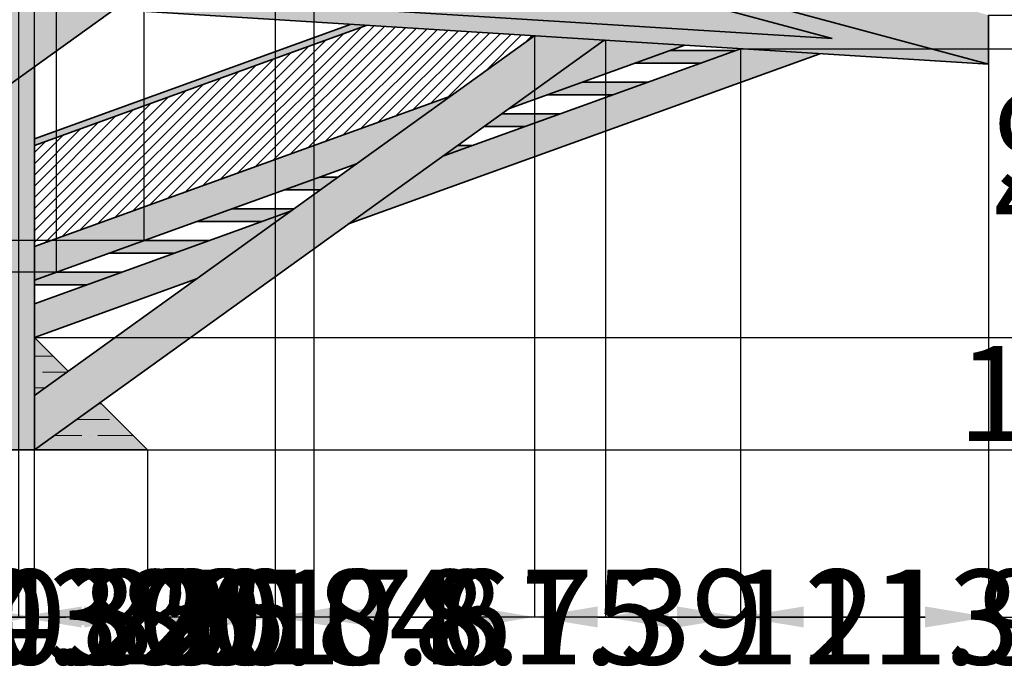
# Model space of a CAD drawing. Units: millimetres. Extents: x -504 to 6314, y 1290 to 4335.
# Tile 6 of 9: x 3796 to 5350, y 1290 to 2332. Entities that reach past the tile are written whole.
import ezdxf

# ---------------------------------------------------------------- set-up
doc = ezdxf.new("R2010")
doc.units = ezdxf.units.MM
doc.header["$MEASUREMENT"] = 0
for name, color, linetype, lineweight in [('A-ANNO-DIMS', 2, 'Continuous', 18), ('A-ELEV', 7, 'Continuous', 35), ('A-ELEV-PATT', 8, 'Continuous', 13)]:
    doc.layers.add(name, color=color, linetype=linetype, lineweight=lineweight)
doc.styles.get("Standard").update_dxf_attribs({"font": 'arial.ttf'})
doc.dimstyles.get("Standard").update_dxf_attribs({"dimtxt": 150, "dimasz": 100, "dimexe": 0.18, "dimexo": 0.0625, "dimgap": 0.09, "dimtad": 0, "dimtih": 1, "dimtoh": 1, "dimdec": 0, "dimzin": 0, "dimdsep": 46, "dimtxsty": 'Standard', "dimcen": 0.09, "dimadec": 0, "dimazin": 0, "dimtfac": 1, "dimtdec": 0, "dimtofl": 0, "dimtmove": 0, "dimatfit": 3, "dimfxl": 1, "dimtolj": 1, "dimtzin": 0, "dimarcsym": 0})
pattern_1 = [(50, (0, 0), (71.726, -6.2752), [7.5, -82.5]), (355, (0, 0), (-13.8751, 75.2192), [6, -66]), (100.4514, (5.98, -0.52), (57.8509, 68.944), [6.374, -70.1142]), (46.1842, (0, 20), (106.7241, -16.5519), [11.25, -123.75]), (96.6356, (8.89, 18.62), (93.4662, 97.4119), [9.561, -105.1714]), (351.1842, (0, 20), (93.4662, 97.4119), [9, -99]), (21, (10, 15), (59.6907, -40.2619), [7.5, -82.5]), (326, (10, 15), (24.3315, 72.515), [6, -66]), (71.4514, (14.974, 11.645), (84.0222, 32.2531), [6.374, -70.1142]), (37.5, (0, 0), (1.21599, 33.28939), [0, -65.2, 0, -67, 0, -66.25]), (7.5, (0, 0), (26.30695, 39.44117), [0, -38.2, 0, -63.7, 0, -25.25]), (327.5, (-22.3, 0), (53.38224, -2.25549), [0, -25, 0, -78, 0, -103.5]), (317.5, (-32.3, 0), (58.3186, 10.0105), [0, -32.5, 0, -51.8, 0, -73.5])]

# ---------------------------------------------------------------- blocks, each defined once
blk = doc.blocks.new('*D1')
at = {"layer": 'A-ANNO-DIMS', "color": 0, "lineweight": -2, "transparency": 16777216}
for p, q in [((5324.8, 2261.1), (5324.8, 1387.9)), ((72.8, 1652.1), (72.8, 1387.9)), ((172.8, 1388.1), (2475.5, 1388.1)), ((5224.8, 1388.1), (2922.1, 1388.1))]:
    blk.add_line(p, q, dxfattribs=at)
at = {"layer": 'A-ANNO-DIMS', "color": 0, "transparency": 16777216}
for points in [[(172.8, 1404.8), (172.8, 1371.5), (72.8, 1388.1)], [(5224.8, 1404.8), (5224.8, 1371.5), (5324.8, 1388.1)]]:
    blk.add_solid(points, dxfattribs=at)
at = {"layer": 'Defpoints', "color": 0, "transparency": 16777216}
for p in [(5324.8, 2261.2), (72.8, 1652.1), (5324.8, 1388.1)]:
    blk.add_point(p, dxfattribs=at)
at = {"layer": 'A-ANNO-DIMS', "color": 0, "transparency": 16777216, "insert": (2698.8, 1388.1), "char_height": 150, "attachment_point": 5}
blk.add_mtext('\\A1;5252', dxfattribs=at)
blk = doc.blocks.new('*D5')
at = {"layer": 'A-ANNO-DIMS', "color": 0, "lineweight": -2, "transparency": 16777216}
for p, q in [((4260.1, 2625.8), (5589, 2625.8)), ((5588.8, 2525.8), (5588.8, 2215.7)), ((5588.8, 1752.1), (5588.8, 2062.2)), ((72.9, 1652.1), (5589, 1652.1))]:
    blk.add_line(p, q, dxfattribs=at)
at = {"layer": 'A-ANNO-DIMS', "color": 0, "transparency": 16777216}
for points in [[(5572.1, 2525.8), (5605.5, 2525.8), (5588.8, 2625.8)], [(5572.1, 1752.1), (5605.5, 1752.1), (5588.8, 1652.1)]]:
    blk.add_solid(points, dxfattribs=at)
at = {"layer": 'Defpoints', "color": 0, "transparency": 16777216}
for p in [(4260, 2625.8), (5588.8, 2625.8), (72.8, 1652.1)]:
    blk.add_point(p, dxfattribs=at)
at = {"layer": 'A-ANNO-DIMS', "color": 0, "transparency": 16777216, "insert": (5588.8, 2138.9), "char_height": 150, "attachment_point": 5}
blk.add_mtext('\\A1;973.6', dxfattribs=at)
blk = doc.blocks.new('*D38')
at = {"layer": 'A-ANNO-DIMS', "color": 0, "lineweight": -2, "transparency": 16777216}
for p, q in [((2963.6, 2625.7), (2963.6, 1387.9)), ((3407.8, 2625.7), (3407.8, 1387.9)), ((3063.6, 1388.1), (3307.8, 1388.1)), ((3407.8, 1388.1), (3507.8, 1388.1))]:
    blk.add_line(p, q, dxfattribs=at)
at = {"layer": 'A-ANNO-DIMS', "color": 0, "transparency": 16777216}
for points in [[(3063.6, 1404.8), (3063.6, 1371.5), (2963.6, 1388.1)], [(3307.8, 1404.8), (3307.8, 1371.5), (3407.8, 1388.1)]]:
    blk.add_solid(points, dxfattribs=at)
at = {"layer": 'Defpoints', "color": 0, "transparency": 16777216}
for p in [(2963.6, 2625.8), (3407.8, 2625.8), (3407.8, 1388.1)]:
    blk.add_point(p, dxfattribs=at)
at = {"layer": 'A-ANNO-DIMS', "color": 0, "transparency": 16777216, "insert": (3763.2, 1388.1), "char_height": 150, "attachment_point": 5}
blk.add_mtext('\\A1;444.2', dxfattribs=at)
blk = doc.blocks.new('*D39')
at = {"layer": 'A-ANNO-DIMS', "color": 0, "lineweight": -2, "transparency": 16777216}
for p, q in [((3407.8, 2625.7), (3407.8, 1387.9)), ((3768.6, 2625.7), (3768.6, 1387.9)), ((3507.8, 1388.1), (3668.6, 1388.1)), ((3768.6, 1388.1), (3868.6, 1388.1))]:
    blk.add_line(p, q, dxfattribs=at)
at = {"layer": 'A-ANNO-DIMS', "color": 0, "transparency": 16777216}
for points in [[(3507.8, 1404.8), (3507.8, 1371.5), (3407.8, 1388.1)], [(3668.6, 1404.8), (3668.6, 1371.5), (3768.6, 1388.1)]]:
    blk.add_solid(points, dxfattribs=at)
at = {"layer": 'Defpoints', "color": 0, "transparency": 16777216}
for p in [(3407.8, 2625.8), (3768.6, 2625.8), (3768.6, 1388.1)]:
    blk.add_point(p, dxfattribs=at)
at = {"layer": 'A-ANNO-DIMS', "color": 0, "transparency": 16777216, "insert": (4179.7, 1388.1), "char_height": 150, "attachment_point": 5}
blk.add_mtext('\\A1;360.84', dxfattribs=at)
blk = doc.blocks.new('*D40')
at = {"layer": 'A-ANNO-DIMS', "color": 0, "lineweight": -2, "transparency": 16777216}
for p, q in [((3768.6, 2625.7), (3768.6, 1387.9)), ((3793.6, 2625.7), (3793.6, 1387.9)), ((3668.6, 1388.1), (3568.6, 1388.1)), ((3893.6, 1388.1), (3993.6, 1388.1))]:
    blk.add_line(p, q, dxfattribs=at)
at = {"layer": 'A-ANNO-DIMS', "color": 0, "transparency": 16777216}
for points in [[(3668.6, 1404.8), (3668.6, 1371.5), (3768.6, 1388.1)], [(3893.6, 1404.8), (3893.6, 1371.5), (3793.6, 1388.1)]]:
    blk.add_solid(points, dxfattribs=at)
at = {"layer": 'Defpoints', "color": 0, "transparency": 16777216}
for p in [(3768.6, 2625.8), (3793.6, 2625.8), (3793.6, 1388.1)]:
    blk.add_point(p, dxfattribs=at)
at = {"layer": 'A-ANNO-DIMS', "color": 0, "transparency": 16777216, "insert": (4103, 1388.1), "char_height": 150, "attachment_point": 5}
blk.add_mtext('\\A1;25', dxfattribs=at)
blk = doc.blocks.new('*D41')
at = {"layer": 'A-ANNO-DIMS', "color": 0, "lineweight": -2, "transparency": 16777216}
for p, q in [((3793.6, 2625.7), (3793.6, 1387.9)), ((3818.6, 2625.7), (3818.6, 1387.9)), ((3693.6, 1388.1), (3593.6, 1388.1)), ((3918.6, 1388.1), (4018.6, 1388.1))]:
    blk.add_line(p, q, dxfattribs=at)
at = {"layer": 'A-ANNO-DIMS', "color": 0, "transparency": 16777216}
for points in [[(3693.6, 1404.8), (3693.6, 1371.5), (3793.6, 1388.1)], [(3918.6, 1404.8), (3918.6, 1371.5), (3818.6, 1388.1)]]:
    blk.add_solid(points, dxfattribs=at)
at = {"layer": 'Defpoints', "color": 0, "transparency": 16777216}
for p in [(3793.6, 2625.8), (3818.6, 2625.8), (3818.6, 1388.1)]:
    blk.add_point(p, dxfattribs=at)
at = {"layer": 'A-ANNO-DIMS', "color": 0, "transparency": 16777216, "insert": (4128, 1388.1), "char_height": 150, "attachment_point": 5}
blk.add_mtext('\\A1;25', dxfattribs=at)
blk = doc.blocks.new('*D42')
at = {"layer": 'A-ANNO-DIMS', "color": 0, "lineweight": -2, "transparency": 16777216}
for p, q in [((3818.6, 2625.7), (3818.6, 1387.9)), ((4198.6, 2625.7), (4198.6, 1387.9)), ((3718.6, 1388.1), (3618.6, 1388.1)), ((4298.6, 1388.1), (4398.6, 1388.1))]:
    blk.add_line(p, q, dxfattribs=at)
at = {"layer": 'A-ANNO-DIMS', "color": 0, "transparency": 16777216}
for points in [[(3718.6, 1404.8), (3718.6, 1371.5), (3818.6, 1388.1)], [(4298.6, 1404.8), (4298.6, 1371.5), (4198.6, 1388.1)]]:
    blk.add_solid(points, dxfattribs=at)
at = {"layer": 'Defpoints', "color": 0, "transparency": 16777216}
for p in [(3818.6, 2625.8), (4198.6, 2625.8), (4198.6, 1388.1)]:
    blk.add_point(p, dxfattribs=at)
at = {"layer": 'A-ANNO-DIMS', "color": 0, "transparency": 16777216, "insert": (4008.6, 1388.1), "char_height": 150, "attachment_point": 5}
blk.add_mtext('\\A1;380', dxfattribs=at)
blk = doc.blocks.new('*D43')
at = {"layer": 'A-ANNO-DIMS', "color": 0, "lineweight": -2, "transparency": 16777216}
for p, q in [((4198.6, 2625.7), (4198.6, 1387.9)), ((4260, 2625.7), (4260, 1387.9)), ((4098.6, 1388.1), (3998.6, 1388.1)), ((4360, 1388.1), (4460, 1388.1))]:
    blk.add_line(p, q, dxfattribs=at)
at = {"layer": 'A-ANNO-DIMS', "color": 0, "transparency": 16777216}
for points in [[(4098.6, 1404.8), (4098.6, 1371.5), (4198.6, 1388.1)], [(4360, 1404.8), (4360, 1371.5), (4260, 1388.1)]]:
    blk.add_solid(points, dxfattribs=at)
at = {"layer": 'Defpoints', "color": 0, "transparency": 16777216}
for p in [(4198.6, 2625.8), (4260, 2625.8), (4260, 1388.1)]:
    blk.add_point(p, dxfattribs=at)
at = {"layer": 'A-ANNO-DIMS', "color": 0, "transparency": 16777216, "insert": (4713.8, 1388.1), "char_height": 150, "attachment_point": 5}
blk.add_mtext('\\A1;61.39', dxfattribs=at)
blk = doc.blocks.new('*D51')
at = {"layer": 'A-ANNO-DIMS', "color": 0, "lineweight": -2, "transparency": 16777216}
for p, q in [((3077, 1702.1), (3077, 1387.9)), ((3397.8, 1702.1), (3397.8, 1387.9)), ((3177, 1388.1), (3297.8, 1388.1)), ((3397.8, 1388.1), (3497.8, 1388.1))]:
    blk.add_line(p, q, dxfattribs=at)
at = {"layer": 'A-ANNO-DIMS', "color": 0, "transparency": 16777216}
for points in [[(3177, 1404.8), (3177, 1371.5), (3077, 1388.1)], [(3297.8, 1404.8), (3297.8, 1371.5), (3397.8, 1388.1)]]:
    blk.add_solid(points, dxfattribs=at)
at = {"layer": 'Defpoints', "color": 0, "transparency": 16777216}
for p in [(3077, 1702.1), (3397.8, 1702.1), (3397.8, 1388.1)]:
    blk.add_point(p, dxfattribs=at)
at = {"layer": 'A-ANNO-DIMS', "color": 0, "transparency": 16777216, "insert": (3751.1, 1388.1), "char_height": 150, "attachment_point": 5}
blk.add_mtext('\\A1;320.8', dxfattribs=at)
blk = doc.blocks.new('*D52')
at = {"layer": 'A-ANNO-DIMS', "color": 0, "lineweight": -2, "transparency": 16777216}
for p, q in [((3397.8, 1702.1), (3397.8, 1387.9)), ((3447.8, 1702.1), (3447.8, 1387.9)), ((3297.8, 1388.1), (3197.8, 1388.1)), ((3547.8, 1388.1), (3647.8, 1388.1))]:
    blk.add_line(p, q, dxfattribs=at)
at = {"layer": 'A-ANNO-DIMS', "color": 0, "transparency": 16777216}
for points in [[(3297.8, 1404.8), (3297.8, 1371.5), (3397.8, 1388.1)], [(3547.8, 1404.8), (3547.8, 1371.5), (3447.8, 1388.1)]]:
    blk.add_solid(points, dxfattribs=at)
at = {"layer": 'Defpoints', "color": 0, "transparency": 16777216}
for p in [(3397.8, 1702.1), (3447.8, 1702.1), (3447.8, 1388.1)]:
    blk.add_point(p, dxfattribs=at)
at = {"layer": 'A-ANNO-DIMS', "color": 0, "transparency": 16777216, "insert": (3755.1, 1388.1), "char_height": 150, "attachment_point": 5}
blk.add_mtext('\\A1;50', dxfattribs=at)
blk = doc.blocks.new('*D53')
at = {"layer": 'A-ANNO-DIMS', "color": 0, "lineweight": -2, "transparency": 16777216}
for p, q in [((3447.8, 1702.1), (3447.8, 1387.9)), ((3768.6, 1702.1), (3768.6, 1387.9)), ((3547.8, 1388.1), (3668.6, 1388.1)), ((3768.6, 1388.1), (3868.6, 1388.1))]:
    blk.add_line(p, q, dxfattribs=at)
at = {"layer": 'A-ANNO-DIMS', "color": 0, "transparency": 16777216}
for points in [[(3547.8, 1404.8), (3547.8, 1371.5), (3447.8, 1388.1)], [(3668.6, 1404.8), (3668.6, 1371.5), (3768.6, 1388.1)]]:
    blk.add_solid(points, dxfattribs=at)
at = {"layer": 'Defpoints', "color": 0, "transparency": 16777216}
for p in [(3447.8, 1702.1), (3768.6, 1702.1), (3768.6, 1388.1)]:
    blk.add_point(p, dxfattribs=at)
at = {"layer": 'A-ANNO-DIMS', "color": 0, "transparency": 16777216, "insert": (4121.9, 1388.1), "char_height": 150, "attachment_point": 5}
blk.add_mtext('\\A1;320.8', dxfattribs=at)
blk = doc.blocks.new('*D54')
at = {"layer": 'A-ANNO-DIMS', "color": 0, "lineweight": -2, "transparency": 16777216}
for p, q in [((3768.6, 1702.1), (3768.6, 1387.9)), ((3818.6, 1652.1), (3818.6, 1387.9)), ((3668.6, 1388.1), (3568.6, 1388.1)), ((3918.6, 1388.1), (4018.6, 1388.1))]:
    blk.add_line(p, q, dxfattribs=at)
at = {"layer": 'A-ANNO-DIMS', "color": 0, "transparency": 16777216}
for points in [[(3668.6, 1404.8), (3668.6, 1371.5), (3768.6, 1388.1)], [(3918.6, 1404.8), (3918.6, 1371.5), (3818.6, 1388.1)]]:
    blk.add_solid(points, dxfattribs=at)
at = {"layer": 'Defpoints', "color": 0, "transparency": 16777216}
for p in [(3768.6, 1702.1), (3818.6, 1652.1), (3818.6, 1388.1)]:
    blk.add_point(p, dxfattribs=at)
at = {"layer": 'A-ANNO-DIMS', "color": 0, "transparency": 16777216, "insert": (4125.9, 1388.1), "char_height": 150, "attachment_point": 5}
blk.add_mtext('\\A1;50', dxfattribs=at)
blk = doc.blocks.new('*D55')
at = {"layer": 'A-ANNO-DIMS', "color": 0, "lineweight": -2, "transparency": 16777216}
for p, q in [((3818.6, 1652.1), (3818.6, 1387.9)), ((3997.4, 1652.1), (3997.4, 1387.9)), ((3718.6, 1388.1), (3618.6, 1388.1)), ((4097.4, 1388.1), (4197.4, 1388.1))]:
    blk.add_line(p, q, dxfattribs=at)
at = {"layer": 'A-ANNO-DIMS', "color": 0, "transparency": 16777216}
for points in [[(3718.6, 1404.8), (3718.6, 1371.5), (3818.6, 1388.1)], [(4097.4, 1404.8), (4097.4, 1371.5), (3997.4, 1388.1)]]:
    blk.add_solid(points, dxfattribs=at)
at = {"layer": 'Defpoints', "color": 0, "transparency": 16777216}
for p in [(3818.6, 1652.1), (3997.4, 1652.1), (3997.4, 1388.1)]:
    blk.add_point(p, dxfattribs=at)
at = {"layer": 'A-ANNO-DIMS', "color": 0, "transparency": 16777216, "insert": (4502.3, 1388.1), "char_height": 150, "attachment_point": 5}
blk.add_mtext('\\A1;178.75', dxfattribs=at)
blk = doc.blocks.new('*D56')
at = {"layer": 'A-ANNO-DIMS', "color": 0, "lineweight": -2, "transparency": 16777216}
for p, q in [((4608.2, 2306), (4608.2, 1387.9)), ((3997.4, 1652.1), (3997.4, 1387.9)), ((3897.4, 1388.1), (3797.4, 1388.1)), ((4708.2, 1388.1), (4808.2, 1388.1))]:
    blk.add_line(p, q, dxfattribs=at)
at = {"layer": 'A-ANNO-DIMS', "color": 0, "transparency": 16777216}
for points in [[(3897.4, 1404.8), (3897.4, 1371.5), (3997.4, 1388.1)], [(4708.2, 1404.8), (4708.2, 1371.5), (4608.2, 1388.1)]]:
    blk.add_solid(points, dxfattribs=at)
at = {"layer": 'Defpoints', "color": 0, "transparency": 16777216}
for p in [(4608.2, 2306.1), (3997.4, 1652.1), (4608.2, 1388.1)]:
    blk.add_point(p, dxfattribs=at)
at = {"layer": 'A-ANNO-DIMS', "color": 0, "transparency": 16777216, "insert": (4302.8, 1388.1), "char_height": 150, "attachment_point": 5}
blk.add_mtext('\\A1;610.8', dxfattribs=at)
blk = doc.blocks.new('*D57')
at = {"layer": 'A-ANNO-DIMS', "color": 0, "lineweight": -2, "transparency": 16777216}
for p, q in [((4608.2, 2306), (4608.2, 1387.9)), ((4720.2, 2299), (4720.2, 1387.9)), ((4508.2, 1388.1), (4408.2, 1388.1)), ((4820.2, 1388.1), (4920.2, 1388.1))]:
    blk.add_line(p, q, dxfattribs=at)
at = {"layer": 'A-ANNO-DIMS', "color": 0, "transparency": 16777216}
for points in [[(4508.2, 1404.8), (4508.2, 1371.5), (4608.2, 1388.1)], [(4820.2, 1404.8), (4820.2, 1371.5), (4720.2, 1388.1)]]:
    blk.add_solid(points, dxfattribs=at)
at = {"layer": 'Defpoints', "color": 0, "transparency": 16777216}
for p in [(4608.2, 2306.1), (4720.2, 2299.1), (4720.2, 1388.1)]:
    blk.add_point(p, dxfattribs=at)
at = {"layer": 'A-ANNO-DIMS', "color": 0, "transparency": 16777216, "insert": (5224.6, 1388.1), "char_height": 150, "attachment_point": 5}
blk.add_mtext('\\A1;111.97', dxfattribs=at)
blk = doc.blocks.new('*D58')
at = {"layer": 'A-ANNO-DIMS', "color": 0, "lineweight": -2, "transparency": 16777216}
for p, q in [((4720.2, 2299), (4720.2, 1387.9)), ((4933.3, 2285.6), (4933.3, 1387.9)), ((4820.2, 1388.1), (4833.3, 1388.1)), ((4933.3, 1388.1), (5033.3, 1388.1))]:
    blk.add_line(p, q, dxfattribs=at)
at = {"layer": 'A-ANNO-DIMS', "color": 0, "transparency": 16777216}
for points in [[(4820.2, 1404.8), (4820.2, 1371.5), (4720.2, 1388.1)], [(4833.3, 1404.8), (4833.3, 1371.5), (4933.3, 1388.1)]]:
    blk.add_solid(points, dxfattribs=at)
at = {"layer": 'Defpoints', "color": 0, "transparency": 16777216}
for p in [(4720.2, 2299.1), (4933.3, 2285.7), (4933.3, 1388.1)]:
    blk.add_point(p, dxfattribs=at)
at = {"layer": 'A-ANNO-DIMS', "color": 0, "transparency": 16777216, "insert": (5346.1, 1388.1), "char_height": 150, "attachment_point": 5}
blk.add_mtext('\\A1;213.13', dxfattribs=at)
blk = doc.blocks.new('*D59')
at = {"layer": 'A-ANNO-DIMS', "color": 0, "lineweight": -2, "transparency": 16777216}
for p, q in [((4933.3, 2285.6), (4933.3, 1387.9)), ((5324.8, 2261.1), (5324.8, 1387.9)), ((5033.3, 1388.1), (5224.8, 1388.1)), ((5324.8, 1388.1), (5424.8, 1388.1))]:
    blk.add_line(p, q, dxfattribs=at)
at = {"layer": 'A-ANNO-DIMS', "color": 0, "transparency": 16777216}
for points in [[(5033.3, 1404.8), (5033.3, 1371.5), (4933.3, 1388.1)], [(5224.8, 1404.8), (5224.8, 1371.5), (5324.8, 1388.1)]]:
    blk.add_solid(points, dxfattribs=at)
at = {"layer": 'Defpoints', "color": 0, "transparency": 16777216}
for p in [(4933.3, 2285.7), (5324.8, 2261.2), (5324.8, 1388.1)]:
    blk.add_point(p, dxfattribs=at)
at = {"layer": 'A-ANNO-DIMS', "color": 0, "transparency": 16777216, "insert": (5678.5, 1388.1), "char_height": 150, "attachment_point": 5}
blk.add_mtext('\\A1;391.5', dxfattribs=at)
blk = doc.blocks.new('*D63')
at = {"layer": 'A-ANNO-DIMS', "color": 0, "lineweight": -2, "transparency": 16777216}
for p, q in [((5588.8, 1929.8), (5588.8, 2029.8)), ((3818.7, 1829.8), (5589, 1829.8)), ((3818.7, 1652.1), (5589, 1652.1)), ((5588.8, 1552.1), (5588.8, 1452.1))]:
    blk.add_line(p, q, dxfattribs=at)
at = {"layer": 'A-ANNO-DIMS', "color": 0, "transparency": 16777216}
for points in [[(5572.1, 1929.8), (5605.5, 1929.8), (5588.8, 1829.8)], [(5572.1, 1552.1), (5605.5, 1552.1), (5588.8, 1652.1)]]:
    blk.add_solid(points, dxfattribs=at)
at = {"layer": 'Defpoints', "color": 0, "transparency": 16777216}
for p in [(3818.6, 1829.8), (5588.8, 1829.8), (3818.6, 1652.1)]:
    blk.add_point(p, dxfattribs=at)
at = {"layer": 'A-ANNO-DIMS', "color": 0, "transparency": 16777216, "insert": (5588.8, 1741), "char_height": 150, "attachment_point": 5}
blk.add_mtext('\\A1;177.65', dxfattribs=at)
blk = doc.blocks.new('*D64')
at = {"layer": 'A-ANNO-DIMS', "color": 0, "lineweight": -2, "transparency": 16777216}
for p, q in [((4933.4, 2285.7), (5589, 2285.7)), ((5588.8, 2185.7), (5588.8, 2134.4)), ((5588.8, 1929.8), (5588.8, 1981.1)), ((3818.7, 1829.8), (5589, 1829.8))]:
    blk.add_line(p, q, dxfattribs=at)
at = {"layer": 'A-ANNO-DIMS', "color": 0, "transparency": 16777216}
for points in [[(5572.1, 2185.7), (5605.5, 2185.7), (5588.8, 2285.7)], [(5572.1, 1929.8), (5605.5, 1929.8), (5588.8, 1829.8)]]:
    blk.add_solid(points, dxfattribs=at)
at = {"layer": 'Defpoints', "color": 0, "transparency": 16777216}
for p in [(4933.3, 2285.7), (5588.8, 2285.7), (3818.6, 1829.8)]:
    blk.add_point(p, dxfattribs=at)
at = {"layer": 'A-ANNO-DIMS', "color": 0, "transparency": 16777216, "insert": (5588.8, 2057.7), "char_height": 150, "attachment_point": 5}
blk.add_mtext('\\A1;455.9', dxfattribs=at)
blk = doc.blocks.new('*D65')
at = {"layer": 'A-ANNO-DIMS', "color": 0, "lineweight": -2, "transparency": 16777216}
for p, q in [((5588.8, 2438.8), (5588.8, 2538.8)), ((5588.8, 2538.8), (5688.8, 2538.8)), ((5324.9, 2338.8), (5589, 2338.8)), ((4933.4, 2285.7), (5589, 2285.7)), ((5588.8, 2185.7), (5588.8, 2085.7))]:
    blk.add_line(p, q, dxfattribs=at)
at = {"layer": 'A-ANNO-DIMS', "color": 0, "transparency": 16777216}
for points in [[(5572.1, 2438.8), (5605.5, 2438.8), (5588.8, 2338.8)], [(5572.1, 2185.7), (5605.5, 2185.7), (5588.8, 2285.7)]]:
    blk.add_solid(points, dxfattribs=at)
at = {"layer": 'Defpoints', "color": 0, "transparency": 16777216}
for p in [(5324.8, 2338.8), (5588.8, 2338.8), (4933.3, 2285.7)]:
    blk.add_point(p, dxfattribs=at)
at = {"layer": 'A-ANNO-DIMS', "color": 0, "transparency": 16777216, "insert": (5941.2, 2538.8), "char_height": 150, "attachment_point": 5}
blk.add_mtext('\\A1;53.12', dxfattribs=at)
blk = doc.blocks.new('*D66')
at = {"layer": 'A-ANNO-DIMS', "color": 0, "lineweight": -2, "transparency": 16777216}
for p, q in [((3753.7, 4236.8), (3653.7, 4236.8)), ((3853.7, 1932.9), (3853.7, 4237)), ((3992.1, 1982.9), (3992.1, 4237)), ((4092.1, 4236.8), (4192.1, 4236.8))]:
    blk.add_line(p, q, dxfattribs=at)
at = {"layer": 'A-ANNO-DIMS', "color": 0, "transparency": 16777216}
for points in [[(3753.7, 4253.4), (3753.7, 4220.1), (3853.7, 4236.8)], [(4092.1, 4253.4), (4092.1, 4220.1), (3992.1, 4236.8)]]:
    blk.add_solid(points, dxfattribs=at)
at = {"layer": 'Defpoints', "color": 0, "transparency": 16777216}
for p in [(3992.1, 4236.8), (3992.1, 1982.8), (3853.7, 1932.8)]:
    blk.add_point(p, dxfattribs=at)
at = {"layer": 'A-ANNO-DIMS', "color": 0, "transparency": 16777216, "insert": (4496.6, 4236.8), "char_height": 150, "attachment_point": 5}
blk.add_mtext('\\A1;138.38', dxfattribs=at)
blk = doc.blocks.new('*D67')
at = {"layer": 'A-ANNO-DIMS', "color": 0, "lineweight": -2, "transparency": 16777216}
for p, q in [((-191.2, 2082.8), (-191.2, 2182.8)), ((-191.2, 2182.8), (-91.2, 2182.8)), ((3992, 1982.8), (-191.3, 1982.8)), ((3853.6, 1932.8), (-191.3, 1932.8)), ((-191.2, 1832.8), (-191.2, 1732.8))]:
    blk.add_line(p, q, dxfattribs=at)
at = {"layer": 'A-ANNO-DIMS', "color": 0, "transparency": 16777216}
for points in [[(-207.8, 2082.8), (-174.5, 2082.8), (-191.2, 1982.8)], [(-207.8, 1832.8), (-174.5, 1832.8), (-191.2, 1932.8)]]:
    blk.add_solid(points, dxfattribs=at)
at = {"layer": 'Defpoints', "color": 0, "transparency": 16777216}
for p in [(-191.2, 1982.8), (3992.1, 1982.8), (3853.7, 1932.8)]:
    blk.add_point(p, dxfattribs=at)
at = {"layer": 'A-ANNO-DIMS', "color": 0, "transparency": 16777216, "insert": (16.1, 2182.8), "char_height": 150, "attachment_point": 5}
blk.add_mtext('\\A1;50', dxfattribs=at)

msp = doc.modelspace()

# ---------------------------------------------------------------- hatches: boundary and pattern name
at = {"layer": 'A-ELEV-PATT'}
h = msp.add_hatch(dxfattribs=at)
h.set_pattern_fill('AR-CONC', color=256, scale=10, style=0)
h.set_pattern_definition(pattern_1)
h.paths.add_polyline_path([(4308.57, 3440.687), (3929.687, 3440.687), (3407.797, 3440.687), (1778.718, 3440.687), (1828.718, 3340.687), (3407.797, 3340.687), (3929.687, 3340.687), (4304.463, 3340.687), (5081.168, 3138.941), (5082.876, 3139.564), (5082.876, 3239.564)])
h.paths.add_polyline_path([(4260.021, 2625.758), (3929.687, 2625.758), (3407.797, 2625.758), (2186.182, 2625.758), (2223.682, 2550.758), (3407.797, 2550.758), (3929.687, 2550.758), (4250.093, 2550.758), (5324.792, 2261.16), (5324.792, 2338.836)])
for points in [[(5324.792, 2261.16), (5324.792, 2338.836), (4260.021, 2625.758), (3929.687, 2625.758), (3407.797, 2625.758), (2186.182, 2625.758), (2223.682, 2550.758), (3407.797, 2550.758), (3929.687, 2550.758), (4250.093, 2550.758)], [(4250.093, 2550.758), (3929.687, 2550.758), (3407.797, 2550.758), (2223.682, 2550.758), (2236.182, 2525.758), (3407.797, 2525.758), (3929.687, 2525.758), (4246.784, 2525.758), (5078.405, 2301.662), (3976.669, 2370.761), (3944.641, 2347.72), (5324.792, 2261.16)], [(4344.074, 2322.669), (4318.999, 2324.241), (3818.634, 2143.445), (3818.634, 2132.813)], [(3922.329, 1726.72), (3872.15, 1776.591), (3818.634, 1738.093), (3818.634, 1652.125)]]:
    msp.add_hatch(color=256, dxfattribs=at).paths.add_polyline_path(points)
h = msp.add_hatch(dxfattribs=at)
h.set_pattern_fill('AR-CONC', color=256, scale=10, style=0)
h.set_pattern_definition(pattern_1)
h.paths.add_polyline_path([(4260.021, 2625.758), (3929.687, 2625.758), (3407.797, 2625.758), (2186.182, 2625.758), (2223.682, 2550.758), (3407.797, 2550.758), (3929.687, 2550.758), (4250.093, 2550.758), (5324.792, 2261.16), (5324.792, 2338.836)])
h = msp.add_hatch(color=256, dxfattribs=at)
h.paths.add_polyline_path([(3076.987, 2525.758), (2403.888, 2525.758), (2840.705, 1652.125), (3076.987, 1822.101)])
h.paths.add_polyline_path([(3922.329, 1726.72), (3818.634, 1652.125), (3997.385, 1652.125)])
h.paths.add_polyline_path([(3818.634, 1829.779), (3818.634, 1738.093), (3872.15, 1776.591)])
h = msp.add_hatch(color=256, dxfattribs=at)
h.paths.add_polyline_path([(4192.131, 2525.758), (4055.138, 2525.758), (2840.705, 1652.125), (2977.698, 1652.125)])
h.paths.add_polyline_path([(4718.141, 2299.208), (4608.219, 2306.102), (3872.15, 1776.591), (3922.329, 1726.72)])
h = msp.add_hatch(color=256, dxfattribs=at)
h.paths.add_polyline_path([(3447.81, 1943.758), (3768.634, 1943.758), (3768.634, 1968.758), (3447.81, 1968.758), (3447.81, 1990.312), (3383.096, 1943.758), (3397.81, 1943.758), (3397.81, 1702.125), (3076.987, 1702.125), (3076.987, 1652.125), (3818.634, 1652.125), (3818.634, 2257.074), (3768.634, 2221.105), (3768.634, 1702.125), (3447.81, 1702.125)])
h.paths.add_polyline_path([(3650.62, 2234.758), (3447.81, 2234.758), (3447.81, 2475.758), (3768.634, 2475.758), (3768.634, 2319.654), (3818.634, 2355.623), (3818.634, 2525.758), (3407.797, 2525.758), (3076.987, 2525.758), (3076.987, 2475.758), (3397.81, 2475.758), (3397.81, 2234.758), (3076.987, 2234.758), (3076.987, 2209.758), (3397.81, 2209.758), (3397.81, 2052.893), (3447.81, 2088.862), (3447.81, 2209.758), (3615.868, 2209.758)])
h.paths.add_polyline_path([(3280.855, 1968.758), (3076.987, 1968.758), (3076.987, 1943.758), (3246.103, 1943.758)], flags=17)
h.paths.add_polyline_path([(3768.634, 2221.105), (3752.861, 2209.758), (3768.634, 2209.758)], flags=17)
h = msp.add_hatch(color=256, dxfattribs=at)
h.set_gradient(color1=(99, 100, 102), color2=(0, 0, 0), name='CYLINDER')
h.paths.add_polyline_path([(5078.405, 2301.662), (4246.784, 2525.758), (4192.131, 2525.758), (3976.669, 2370.761)])
h.paths.add_polyline_path([(4055.138, 2525.758), (3929.687, 2525.758), (3818.634, 2525.758), (3818.634, 2380.672), (3850.662, 2378.664)])
h = msp.add_hatch(dxfattribs=at)
h.set_pattern_fill('ANSI31', color=256, scale=100, style=0)
h.paths.add_polyline_path([(4475.606, 2210.704), (4608.219, 2306.102), (4344.074, 2322.669), (3818.634, 2132.813), (3818.634, 1973.321)])
h = msp.add_hatch(color=256, dxfattribs=at)
h.paths.add_polyline_path([(4327.124, 2103.889), (4475.606, 2210.704), (3818.634, 1973.321), (3818.634, 1920.157)])
h.paths.add_polyline_path([(4845.566, 2291.216), (4720.193, 2299.079), (4715.71, 2297.46), (4567.228, 2190.645)])
h = msp.add_hatch(color=256, dxfattribs=at)
h.paths.add_polyline_path([(5058.7, 2277.849), (4933.327, 2285.712), (4463.29, 2115.875), (4314.808, 2009.06)])
h.paths.add_polyline_path([(4223.186, 2029.119), (3818.634, 1882.943), (3818.634, 1829.779), (4074.704, 1922.304)])
h = msp.add_hatch(color=256, dxfattribs=at)
h.set_gradient(color1=(99, 100, 102), color2=(0, 0, 0), name='CYLINDER')
h.paths.add_polyline_path([(4822.358, 2282.831), (4767.007, 2262.831), (4870.001, 2262.831), (4925.352, 2282.831)])
h = msp.add_hatch(color=256, dxfattribs=at)
h.set_gradient(color1=(99, 100, 102), color2=(0, 0, 0), name='CYLINDER')
h.paths.add_polyline_path([(4683.98, 2232.831), (4628.628, 2212.831), (4731.623, 2212.831), (4786.974, 2232.831)])
h = msp.add_hatch(color=256, dxfattribs=at)
h.set_gradient(color1=(99, 100, 102), color2=(0, 0, 0), name='CYLINDER')
h.paths.add_polyline_path([(4556.365, 2182.831), (4528.563, 2162.831), (4593.244, 2162.831), (4648.595, 2182.831)])
h = msp.add_hatch(color=256, dxfattribs=at)
h.set_gradient(color1=(99, 100, 102), color2=(0, 0, 0), name='CYLINDER')
h.paths.add_polyline_path([(4556.365, 2182.831), (4528.563, 2162.831), (4593.244, 2162.831), (4648.595, 2182.831)])
h = msp.add_hatch(color=256, dxfattribs=at)
h.set_gradient(color1=(99, 100, 102), color2=(0, 0, 0), name='CYLINDER')
h.paths.add_polyline_path([(4510.217, 2132.831), (4486.861, 2132.831), (4463.29, 2115.875)])
h = msp.add_hatch(color=256, dxfattribs=at)
h.set_gradient(color1=(99, 100, 102), color2=(0, 0, 0), name='CYLINDER')
h.paths.add_polyline_path([(4213.493, 2062.831), (4270.049, 2062.831), (4297.851, 2082.831), (4268.844, 2082.831)])
h = msp.add_hatch(color=256, dxfattribs=at)
h.set_gradient(color1=(99, 100, 102), color2=(0, 0, 0), name='CYLINDER')
h.paths.add_polyline_path([(4130.466, 2032.831), (4075.114, 2012.831), (4178.108, 2012.831), (4223.186, 2029.119), (4228.346, 2032.831)])
h = msp.add_hatch(color=256, dxfattribs=at)
h.set_gradient(color1=(99, 100, 102), color2=(0, 0, 0), name='CYLINDER')
h.paths.add_polyline_path([(4039.73, 1962.831), (4095.081, 1982.831), (3992.087, 1982.831), (3936.736, 1962.831)])
h = msp.add_hatch(color=256, dxfattribs=at)
h.set_gradient(color1=(99, 100, 102), color2=(0, 0, 0), name='CYLINDER')
h.paths.add_polyline_path([(3901.351, 1912.831), (3956.703, 1932.831), (3853.708, 1932.831), (3818.634, 1920.157), (3818.634, 1912.831)])
h = msp.add_hatch(dxfattribs=at)
h.set_pattern_fill('ANSI36', color=256, scale=200, angle=135, style=0)
h.paths.add_polyline_path([(3076.987, 1723.551), (2977.698, 1652.125), (3076.987, 1652.125)])
h.paths.add_polyline_path([(3922.329, 1726.72), (3818.634, 1652.125), (3997.385, 1652.125)])
h.paths.add_polyline_path([(3818.634, 1829.779), (3818.634, 1738.093), (3872.15, 1776.591)])

# ---------------------------------------------------------------- linework, layer by layer
at = {"layer": 'A-ELEV'}
for p, q in [((4250.093, 2550.758), (5324.792, 2261.16)), ((2977.698, 1652.125), (4192.131, 2525.758)), ((4246.784, 2525.758), (5078.405, 2301.662)), ((5078.405, 2301.662), (3976.669, 2370.761)), ((5324.792, 2261.16), (3944.641, 2347.72)), ((5324.792, 2261.16), (5324.792, 2338.836)), ((4318.999, 2324.241), (3818.634, 2143.445)), ((4344.074, 2322.669), (3818.634, 2132.813)), ((3818.634, 1738.093), (4608.219, 2306.102)), ((3818.634, 1652.125), (4718.141, 2299.208)), ((3818.634, 1652.125), (4718.141, 2299.208)), ((4933.327, 2285.712), (4463.29, 2115.875)), ((4845.566, 2291.216), (4567.228, 2190.645)), ((4720.193, 2299.079), (4715.71, 2297.46)), ((5058.7, 2277.849), (4314.808, 2009.06)), ((4822.358, 2282.831), (4925.352, 2282.831)), ((3818.634, 1652.125), (3818.634, 2257.074)), ((4767.007, 2262.831), (4870.001, 2262.831)), ((4684.485, 2232.831), (4786.974, 2232.831)), ((4475.606, 2210.704), (3818.634, 1973.321)), ((4628.628, 2212.831), (4731.623, 2212.831)), ((4556.365, 2182.831), (4648.595, 2182.831)), ((4528.563, 2162.831), (4593.244, 2162.831)), ((4486.861, 2132.831), (4510.217, 2132.831)), ((4327.124, 2103.889), (3818.634, 1920.157)), ((4268.844, 2082.831), (4297.851, 2082.831)), ((4213.493, 2062.831), (4270.049, 2062.831)), ((4223.186, 2029.119), (3818.634, 1882.943)), ((4130.466, 2032.831), (4228.346, 2032.831)), ((4075.114, 2012.831), (4178.108, 2012.831)), ((3992.087, 1982.831), (4095.081, 1982.831)), ((3936.736, 1962.831), (4039.73, 1962.831)), ((3853.708, 1932.831), (3956.703, 1932.831)), ((4074.704, 1922.304), (3818.634, 1829.779)), ((3818.634, 1912.831), (3901.351, 1912.831)), ((3818.634, 1829.779), (3872.15, 1776.591)), ((3922.329, 1726.72), (3997.385, 1652.125)), ((3076.987, 1652.125), (3818.634, 1652.125)), ((3818.634, 1652.125), (3997.385, 1652.125))]:
    msp.add_line(p, q, dxfattribs=at)

# ---------------------------------------------------------------- dimensions: what is measured, and where the dimension line sits
at = {"layer": 'A-ANNO-DIMS'}
for base, p1, p2, override, picture, middle in [((3992.087, 4236.781), (3853.708, 1932.831), (3992.087, 1982.831), {"dimdec": 2, "dimlfac": 1, "dimrnd": 0, "dimzin": 0, "dimdsep": 46, "dimlunit": 2}, '*D66', (4496.628, 4236.781)), ((3407.797, 1388.125), (2963.634, 2625.758), (3407.797, 2625.758), {"dimdec": 1, "dimlfac": 1, "dimrnd": 0, "dimzin": 0, "dimdsep": 46, "dimlunit": 2}, '*D38', (3763.224, 1388.125)), ((3768.634, 1388.125), (3407.797, 2625.758), (3768.634, 2625.758), {"dimdec": 2, "dimlfac": 1, "dimrnd": 0, "dimzin": 0, "dimdsep": 46, "dimlunit": 2}, '*D39', (4179.723, 1388.125)), ((3793.634, 1388.125), (3768.634, 2625.758), (3793.634, 2625.758), {"dimdec": 0, "dimlfac": 1, "dimrnd": 0, "dimzin": 0, "dimdsep": 46, "dimlunit": 2}, '*D40', (4103.001, 1388.125)), ((3818.634, 1388.125), (3793.634, 2625.758), (3818.634, 2625.758), {"dimdec": 0, "dimlfac": 1, "dimrnd": 0, "dimzin": 0, "dimdsep": 46, "dimlunit": 2}, '*D41', (4128.001, 1388.125)), ((4198.634, 1388.125), (3818.634, 2625.758), (4198.634, 2625.758), {"dimdec": 0, "dimlfac": 1, "dimrnd": 0, "dimzin": 0, "dimdsep": 46, "dimlunit": 2}, '*D42', (4008.634, 1388.125)), ((4260.021, 1388.125), (4198.634, 2625.758), (4260.021, 2625.758), {"dimdec": 2, "dimlfac": 1, "dimrnd": 0, "dimzin": 0, "dimdsep": 46, "dimlunit": 2}, '*D43', (4713.761, 1388.125)), ((4608.219, 1388.125), (3997.385, 1652.125), (4608.219, 2306.102), {"dimdec": 1, "dimlfac": 1, "dimrnd": 0, "dimzin": 0, "dimdsep": 46, "dimlunit": 2}, '*D56', (4302.802, 1388.125)), ((4720.193, 1388.125), (4608.219, 2306.102), (4720.193, 2299.079), {"dimdec": 2, "dimlfac": 1, "dimrnd": 0, "dimzin": 0, "dimdsep": 46, "dimlunit": 2}, '*D57', (5224.58, 1388.125)), ((4933.327, 1388.125), (4720.193, 2299.079), (4933.327, 2285.712), {"dimdec": 2, "dimlfac": 1, "dimrnd": 0, "dimzin": 0, "dimdsep": 46, "dimlunit": 2}, '*D58', (5346.053, 1388.125)), ((5324.792, 1388.125), (4933.327, 2285.712), (5324.792, 2261.16), {"dimdec": 1, "dimlfac": 1, "dimrnd": 0, "dimzin": 0, "dimdsep": 46, "dimlunit": 2}, '*D59', (5678.48, 1388.125)), ((5324.792, 1388.125), (72.835, 1652.125), (5324.792, 2261.16), {"dimdec": 0, "dimlfac": 1, "dimrnd": 0, "dimzin": 0, "dimdsep": 46, "dimlunit": 2}, '*D1', (2698.814, 1388.125)), ((3397.81, 1388.125), (3076.987, 1702.125), (3397.81, 1702.125), {"dimdec": 1, "dimlfac": 1, "dimrnd": 0, "dimzin": 0, "dimdsep": 46, "dimlunit": 2}, '*D51', (3751.089, 1388.125)), ((3447.81, 1388.125), (3397.81, 1702.125), (3447.81, 1702.125), {"dimdec": 0, "dimlfac": 1, "dimrnd": 0, "dimzin": 0, "dimdsep": 46, "dimlunit": 2}, '*D52', (3755.08, 1388.125)), ((3768.634, 1388.125), (3447.81, 1702.125), (3768.634, 1702.125), {"dimdec": 1, "dimlfac": 1, "dimrnd": 0, "dimzin": 0, "dimdsep": 46, "dimlunit": 2}, '*D53', (4121.913, 1388.125)), ((3818.634, 1388.125), (3768.634, 1702.125), (3818.634, 1652.125), {"dimdec": 0, "dimlfac": 1, "dimrnd": 0, "dimzin": 0, "dimdsep": 46, "dimlunit": 2}, '*D54', (4125.903, 1388.125)), ((3997.385, 1388.125), (3818.634, 1652.125), (3997.385, 1652.125), {"dimdec": 2, "dimlfac": 1, "dimrnd": 0, "dimzin": 0, "dimdsep": 46, "dimlunit": 2}, '*D55', (4502.335, 1388.125))]:
    dim = msp.add_linear_dim(base=base, p1=p1, p2=p2, dimstyle='Standard', override=override, dxfattribs=at)
    dim.commit()
    dim.dimension.update_dxf_attribs({"geometry": picture, "text_midpoint": middle})
for base, p1, p2, override, picture, middle in [((5588.792, 2338.836), (4933.327, 2285.712), (5324.792, 2338.836), {"dimdec": 2, "dimlfac": 1, "dimrnd": 0, "dimzin": 0, "dimdsep": 46, "dimlunit": 2}, '*D65', (5941.201, 2538.836)), ((5588.792, 2625.758), (72.835, 1652.125), (4260.021, 2625.758), {"dimdec": 1, "dimlfac": 1, "dimrnd": 0, "dimzin": 0, "dimdsep": 46, "dimlunit": 2}, '*D5', (5588.792, 2138.941)), ((5588.792, 2285.712), (3818.634, 1829.779), (4933.327, 2285.712), {"dimdec": 1, "dimlfac": 1, "dimrnd": 0, "dimzin": 0, "dimdsep": 46, "dimlunit": 2}, '*D64', (5588.792, 2057.745)), ((-191.165, 1982.831), (3853.708, 1932.831), (3992.087, 1982.831), {"dimdec": 0, "dimlfac": 1, "dimrnd": 0, "dimzin": 0, "dimdsep": 46, "dimlunit": 2}, '*D67', (16.104, 2182.831)), ((5588.792, 1829.779), (3818.634, 1652.125), (3818.634, 1829.779), {"dimdec": 2, "dimlfac": 1, "dimrnd": 0, "dimzin": 0, "dimdsep": 46, "dimlunit": 2}, '*D63', (5588.792, 1740.952))]:
    dim = msp.add_linear_dim(base=base, p1=p1, p2=p2, angle=90, dimstyle='Standard', override=override, dxfattribs=at)
    dim.commit()
    dim.dimension.update_dxf_attribs({"geometry": picture, "text_midpoint": middle})

doc.saveas('drawing.dxf')
